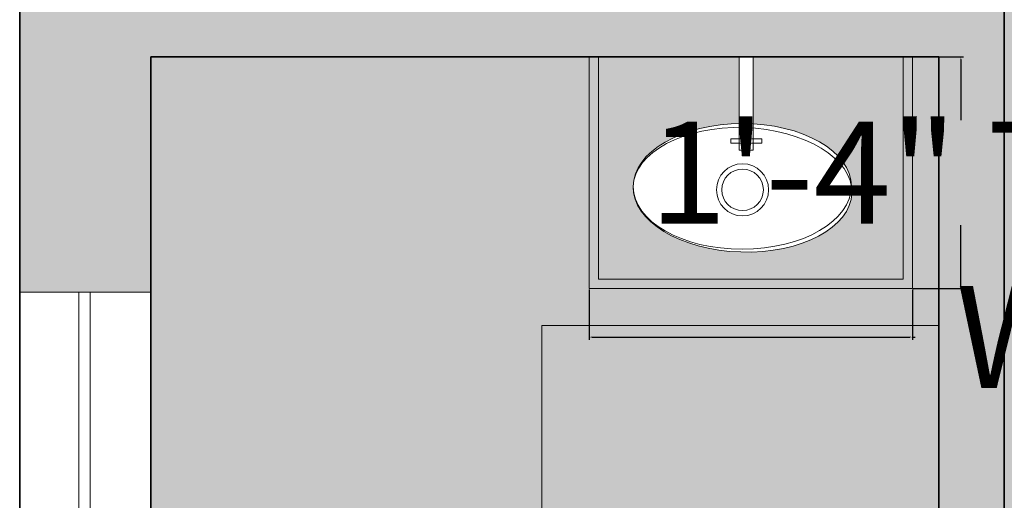
# Model space of a CAD drawing. Units: inches. Extents: x 1316 to 1777, y 813 to 1650.
# Tile 6 of 22: x 1377 to 1445, y 1335 to 1368. Entities that reach past the tile are written whole.
import ezdxf

# ---------------------------------------------------------------- set-up
doc = ezdxf.new("R2010")
doc.units = ezdxf.units.IN
doc.header["$MEASUREMENT"] = 0
for name, color, linetype, lineweight in [('A-ANNO-DIMS', 2, 'Continuous', 18), ('A-FLOR-CASE', 23, 'Continuous', 18), ('A-FLOR-CASE-PATT', 252, 'Continuous', 13), ('A-FLOR-FIXT', 8, 'Continuous', 18), ('A-FLOR-FIXT-PATT', 23, 'Continuous', 13), ('A-WALL-PATT', 250, 'Continuous', 13), ('walls', 250, 'Continuous', 35), ('windows', 141, 'Continuous', 18)]:
    doc.layers.add(name, color=color, linetype=linetype, lineweight=lineweight)
doc.layers.add('A-FLOR-PATT', color=254, linetype='Continuous', lineweight=13, true_color=0xfeeab9)
doc.styles.get("Standard").update_dxf_attribs({"font": 'arial.ttf'})
doc.dimstyles.get("Standard").update_dxf_attribs({"dimtxt": 7, "dimasz": 0.18, "dimexe": 0.18, "dimexo": 0.0625, "dimgap": 0.09, "dimtad": 0, "dimtih": 1, "dimtoh": 1, "dimzin": 0, "dimdsep": 46, "dimlunit": 3, "dimtxsty": 'Standard', "dimcen": 0.09, "dimadec": 0, "dimazin": 0, "dimtfac": 1, "dimtofl": 0, "dimtmove": 0, "dimatfit": 3, "dimfxl": 1, "dimtolj": 1, "dimtzin": 0, "dimarcsym": 0})

# ---------------------------------------------------------------- blocks, each defined once
blk = doc.blocks.new('BASIN-WALL-MOUNT')
for p, q in [((1.14249530725e-05, 15.91430092696169), (1.14249530725e-05, 0.0001979362143629)), ((0.6273383677073526, 15.91430092696169), (0.6273383677073526, 0.658722965959214)), ((10.28959255677932, 9.494232840090262), (10.28959255677932, 15.91430092696191)), ((11.23449039203865, 9.494232840090262), (11.23449039203865, 15.91430092696191)), ((21.53012297768464, 0.658722965959214), (21.53012297768464, 15.91430092696169)), ((22.15516133140068, 0.0001979362143629), (22.15516133140068, 15.91430092696191)), ((9.712388442003657, 10.28665921264746), (11.83648863631629, 10.28665921264746)), ((9.71238844200343, 9.99122808939319), (9.712388442003657, 10.28665921264746)), ((11.83648863631629, 10.28665921264746), (11.83648863631629, 9.99122808939319)), ((11.83648863631629, 9.99122808939319), (9.71238844200343, 9.99122808939319)), ((10.28959255677932, 9.494232840090262), (11.23449039203865, 9.494232840090262)), ((1.14249530725e-05, 0.0001979362143629), (22.15516133140068, 0.0001979362143629)), ((0.6273383677073526, 0.658722965959214), (21.53012297768464, 0.658722965959214))]:
    blk.add_line(p, q)
for radius in [1.786721855987963, 1.786721855987973, 1.426627914243592, 1.426627914243628, 1.42662769250472, 1.426627377330596]:
    blk.add_circle((10.51220414605791, 6.779323088421051), radius)
blk.add_ellipse((10.49584697256341, 7.01803233833516), major_axis=(-7.480193534640648, -0.0164125256646912), ratio=0.5765346257282574)
blk = doc.blocks.new('*D36')
at = {"layer": 'A-ANNO-DIMS', "color": 0, "lineweight": -2, "transparency": 16777216}
for p, q in [((1416.108011424953, 1349.392697936214), (1416.108011424953, 1345.951925450247)), ((1438.2631613314, 1349.392697936214), (1438.2631613314, 1345.951925450247)), ((1416.288011424953, 1346.131925450247), (1438.0831613314, 1346.131925450247)), ((1438.2631613314, 1346.131925450247), (1438.443161331401, 1346.131925450247))]:
    blk.add_line(p, q, dxfattribs=at)
at = {"layer": 'A-ANNO-DIMS', "color": 0, "transparency": 16777216}
for points in [[(1416.288011424953, 1346.161925450247), (1416.288011424953, 1346.101925450247), (1416.108011424953, 1346.131925450247)], [(1438.0831613314, 1346.161925450247), (1438.0831613314, 1346.101925450247), (1438.2631613314, 1346.131925450247)]]:
    blk.add_solid(points, dxfattribs=at)
at = {"layer": 'Defpoints', "color": 0, "transparency": 16777216}
for p in [(1416.108011424953, 1349.455197936214), (1438.2631613314, 1349.455197936214), (1438.2631613314, 1346.131925450247)]:
    blk.add_point(p, dxfattribs=at)
at = {"layer": 'A-ANNO-DIMS', "color": 0, "transparency": 16777216, "insert": (1493.434934864825, 1346.131925450247), "char_height": 7, "attachment_point": 5}
blk.add_mtext('\\A1;WALL BASIN 1\'-10" TYP.', dxfattribs=at)
blk = doc.blocks.new('*D37')
at = {"layer": 'A-ANNO-DIMS', "color": 0, "lineweight": -2, "transparency": 16777216}
for p, q in [((1438.325661331401, 1365.369300926962), (1441.766433817369, 1365.369300926962)), ((1441.586433817368, 1365.189300926962), (1441.586433817368, 1361.018961573471)), ((1441.586433817368, 1349.635197936215), (1441.586433817368, 1353.805537289705)), ((1438.325661331401, 1349.455197936215), (1441.766433817369, 1349.455197936215))]:
    blk.add_line(p, q, dxfattribs=at)
at = {"layer": 'A-ANNO-DIMS', "color": 0, "transparency": 16777216}
for points in [[(1441.556433817369, 1365.189300926962), (1441.616433817368, 1365.189300926962), (1441.586433817368, 1365.369300926962)], [(1441.556433817369, 1349.635197936215), (1441.616433817368, 1349.635197936215), (1441.586433817368, 1349.455197936215)]]:
    blk.add_solid(points, dxfattribs=at)
at = {"layer": 'Defpoints', "color": 0, "transparency": 16777216}
for p in [(1438.263161331401, 1365.369300926962), (1441.586433817368, 1365.369300926962), (1438.263161331401, 1349.455197936215)]:
    blk.add_point(p, dxfattribs=at)
at = {"layer": 'A-ANNO-DIMS', "color": 0, "transparency": 16777216, "insert": (1441.586433817368, 1357.412249431588), "char_height": 7, "attachment_point": 5}
blk.add_mtext('\\A1;1\'-4" TYP.', dxfattribs=at)

msp = doc.modelspace()

# ---------------------------------------------------------------- hatches: boundary and pattern name
at = {"layer": 'A-FLOR-CASE-PATT'}
h = msp.add_hatch(color=256, dxfattribs=at)
h.dxf.hatch_style = 1
h.paths.add_polyline_path([(1412.858226839809, 1346.928610372446), (1440.064450217018, 1346.928610372446), (1440.064450217018, 1365.369300926962), (1438.2631613314, 1365.369300926962), (1438.2631613314, 1349.455197936214), (1416.108011424953, 1349.455197936214), (1416.108011424953, 1365.369300926962), (1386.064450217018, 1365.369300926962), (1386.064450217018, 1245.369300926962), (1412.858226839809, 1245.369300926962)])
h.paths.add_polyline_path([(1409.310422891292, 1332.514765372921, -0.4142135623730951), (1410.210422891292, 1331.614765372921), (1410.210422891292, 1311.814765372921, -0.414213562373094), (1409.310422891292, 1310.914765372921), (1389.51042289129, 1310.914765372921, -0.4142135623730959), (1388.61042289129, 1311.814765372921), (1388.61042289129, 1331.614765372921, -0.4142135623730951), (1389.51042289129, 1332.514765372921)], flags=16)
h.paths.add_polyline_path([(1395.986900854525, 1329.42133126595), (1396.276368249055, 1329.76630507332, -0.0171905986958355), (1396.448908786205, 1329.621893017294), (1396.159470211814, 1329.276953556429, -0.2116405901053515), (1397.086205654243, 1327.18561240685, -0.2564460938474173), (1395.778569555149, 1324.8037474367), (1396.003749512095, 1324.413724310425, -0.0171906504505625), (1395.809203446643, 1324.300687980197), (1395.584072921188, 1324.69062548862, -0.550570801787435), (1391.442799396982, 1327.059740487748), (1390.992413104956, 1327.059740487748, -0.0171907290098312), (1390.991493340996, 1327.284740487748), (1391.441732803486, 1327.284740487748, -0.6105283005508269)], flags=0)
h.paths.add_polyline_path([(1395.838098786515, 1327.18561240685, -1), (1392.688098786514, 1327.18561240685, -1)], flags=0)
h.paths.add_polyline_path([(1394.263098786514, 1328.310612406851, -1), (1394.263098786514, 1326.06061240685, -1)], flags=0)
h.paths.add_polyline_path([(1394.263098786514, 1327.973112406851, -1), (1394.263098786514, 1326.39811240685, -1)], flags=0)
h.paths.add_polyline_path([(1407.468247061996, 1327.18561240685, -0.9779444631718501), (1401.824840804736, 1327.059740487748), (1401.37445451271, 1327.059740487748, -0.0171907290098312), (1401.373534748749, 1327.284740487748), (1401.823774211239, 1327.284740487748, -0.9825922263687022)], flags=0)
h.paths.add_polyline_path([(1406.220140194268, 1327.18561240685, -1), (1403.070140194268, 1327.18561240685, -1)], flags=0)
h.paths.add_polyline_path([(1404.645140194268, 1328.310612406851, -1), (1404.645140194268, 1326.06061240685, -1)], flags=0)
h.paths.add_polyline_path([(1404.645140194268, 1327.973112406851, -1), (1404.645140194268, 1326.39811240685, -1)], flags=0)
h.paths.add_polyline_path([(1400.91382896134, 1321.714765372921, -1), (1397.907016821244, 1321.714765372921, -1)], flags=0)
h.paths.add_polyline_path([(1396.101714535222, 1318.885415367262), (1396.391181929752, 1319.230389174631, -0.0171905986957908), (1396.563722466901, 1319.085977118605), (1396.274283892511, 1318.74103765774, -0.2116405901053402), (1397.201019334939, 1316.649696508162, -0.2564460938474829), (1395.893383235845, 1314.267831538011), (1396.11856319279, 1313.877808411735, -0.0171906504505387), (1395.924017127339, 1313.764772081509), (1395.698886601884, 1314.154709589932, -0.5505708017872751), (1391.557613077679, 1316.523824589059), (1391.107226785653, 1316.523824589059, -0.0171907290098486), (1391.106307021692, 1316.748824589059), (1391.556546484182, 1316.748824589059, -0.6105283005510082)], flags=0)
h.paths.add_polyline_path([(1395.952912467211, 1316.649696508162, -1), (1392.802912467211, 1316.649696508162, -1)], flags=0)
h.paths.add_polyline_path([(1407.468247061996, 1316.611253873528, -0.9779444631716472), (1401.824840804736, 1316.485381954425), (1401.37445451271, 1316.485381954425, -0.0171907290098486), (1401.373534748749, 1316.710381954425), (1401.823774211239, 1316.710381954425, -0.9825922263688615)], flags=0)
h.paths.add_polyline_path([(1394.377912467211, 1317.774696508162, -0.9999999703822144), (1394.377912467211, 1315.524696508162, -0.9999999703822144)], flags=0)
h.paths.add_polyline_path([(1394.377912467211, 1317.437196508162, -1), (1394.377912467211, 1315.862196508162, -1)], flags=0)
h.paths.add_polyline_path([(1406.220140194268, 1316.611253873528, -1), (1403.070140194268, 1316.611253873528, -1)], flags=0)
h.paths.add_polyline_path([(1404.645140194268, 1315.486253873528, -0.9999999703822144), (1404.645140194268, 1317.736253873528, -0.9999999703822144)], flags=0)
h.paths.add_polyline_path([(1404.645140194268, 1317.398753873528, -1), (1404.645140194268, 1315.823753873528, -1)], flags=0)
h.paths.add_polyline_path([(1409.338253781963, 1302.100142632137, -0.4142135623730951), (1410.838253781963, 1300.600142632137), (1410.838253781963, 1270.600142632137, -0.4142135623730951), (1409.338253781963, 1269.100142632137), (1390.338253781963, 1269.100142632137, -0.4142135623730951), (1388.838253781963, 1270.600142632137), (1388.838253781963, 1300.600142632137, -0.4142135623730951), (1390.338253781963, 1302.100142632137)], flags=16)
h.paths.add_polyline_path([(1395.838253781963, 1300.600142632137), (1406.338253781963, 1300.600142632137, -0.4142135623730951), (1409.338253781963, 1297.600142632137), (1409.338253781963, 1289.600142632137, -0.4142135623730951), (1406.338253781963, 1286.600142632137), (1395.838253781963, 1286.600142632137, -0.4142135623730951), (1392.838253781963, 1289.600142632137), (1392.838253781963, 1297.600142632137, -0.4142135623730951)], flags=0)
h.paths.add_polyline_path([(1400.088253781963, 1293.350142632137, -1), (1397.588253781963, 1293.350142632137, -1)], flags=0)
h.paths.add_polyline_path([(1392.338253781963, 1288.600142632137, -1), (1390.338253781963, 1288.600142632137, -1)], flags=0)
h.paths.add_polyline_path([(1393.037126479862, 1286.524525876857), (1399.01645688764, 1282.033156148475), (1398.51645688764, 1281.167130148475), (1391.719002681245, 1284.064804380225, -0.4631994748411593), (1391.203386694108, 1285.500520483254), (1391.606259694108, 1286.198316483253, -0.4369421512224802)], flags=0)
h.paths.add_polyline_path([(1392.338253781963, 1282.600142632137, -1), (1390.338253781963, 1282.600142632137, -1)], flags=0)
h.paths.add_polyline_path([(1400.088253781963, 1277.850142632137, -1), (1397.588253781963, 1277.850142632137, -1)], flags=0)
at = {"layer": 'A-FLOR-FIXT-PATT'}
h = msp.add_hatch(color=256, dxfattribs=at)
h.dxf.hatch_style = 1
h.paths.add_polyline_path([(1438.2631613314, 1365.369300926962), (1437.638122977684, 1365.369300926962), (1437.638122977684, 1350.113722965959), (1416.735338367707, 1350.113722965959), (1416.735338367707, 1365.369300926962), (1416.108011424953, 1365.369300926962), (1416.108011424953, 1349.455197936214), (1438.2631613314, 1349.455197936214)])
h = msp.add_hatch(color=256, dxfattribs=at)
h.dxf.hatch_style = 1
edge = h.paths.add_edge_path()
edge.add_line((1426.397592556779, 1365.369300926962), (1416.735338367707, 1365.369300926962))
edge.add_line((1416.735338367707, 1365.369300926962), (1416.735338367707, 1350.113722965959))
edge.add_line((1416.735338367707, 1350.113722965959), (1437.638122977684, 1350.113722965959))
edge.add_line((1437.638122977684, 1350.113722965959), (1437.638122977684, 1365.369300926962))
edge.add_line((1437.638122977684, 1365.369300926962), (1427.342490392038, 1365.369300926962))
edge.add_line((1427.342490392038, 1365.369300926962), (1427.342490392038, 1360.765644863863))
edge.add_ellipse((1426.603846972563, 1356.473032338335), major_axis=(-7.480193534640648, -0.0164125256646912), ratio=0.5765346257282575, start_angle=180, end_angle=260.11083298804067, ccw=False)
edge.add_ellipse((1426.620204146058, 1356.234323088421), major_axis=(7.496550708135166, -0.2222967242493548), ratio=0.5689904069289865, start_angle=-180, end_angle=3.6561733604243045, ccw=False)
edge.add_ellipse((1426.603846972563, 1356.473032338335), major_axis=(-7.480193534640648, -0.0164125256646912), ratio=0.5765346257282575, start_angle=272.6136539907866, end_angle=360, ccw=False)
edge.add_line((1426.397592556779, 1360.783698373135), (1426.397592556779, 1365.369300926962))
at = {"layer": 'A-FLOR-PATT'}
h = msp.add_hatch(color=256, dxfattribs=at)
h.dxf.hatch_style = 1
h.paths.add_polyline_path([(1567.673142217696, 1281.369300926962), (1651.673142217696, 1281.369300926962), (1651.673142217696, 1365.369300926962), (1597.673142217696, 1365.369300926962), (1597.673142217696, 1429.869300926962), (1570.345136951899, 1429.869300926962), (1570.345136951899, 1471.869300926962), (1510.345136951899, 1471.869300926962), (1510.345136951899, 1429.869300926962), (1444.564450217018, 1429.869300926962), (1444.564450217018, 1322.882360660317), (1444.564450217018, 1300.087519887597), (1510.564450217018, 1300.087519887597), (1510.564450217018, 1295.093869264817), (1510.564450217018, 1240.869300926962), (1386.064450217018, 1240.869300926962), (1386.064450217018, 1171.184826128129), (1400.961298831769, 1171.184826128129), (1400.961298831769, 1106.74181853581), (1386.064450217018, 1106.74181853581), (1386.064450217018, 1072.869300926962), (1510.564450217018, 1072.869300926962), (1510.564450217018, 1040.172951843256), (1541.068383692007, 1040.172951843256, -0.367085007058701), (1572.764174999282, 1069.546549507821), (1572.764174999282, 1069.578525976929), (1574.225256623933, 1069.578525976929), (1574.225256623933, 1040.172951843256), (1616.037285953149, 1040.172951843256), (1616.037285953149, 1086.627161740109), (1616.037285953149, 1103.704513499145), (1613.066060418845, 1105.234780569291), (1616.037285953149, 1106.685539866415), (1616.037285953149, 1123.869300926962), (1567.673142217696, 1123.869300926962)])
h.paths.add_polyline_path([(1508.987494855724, 1198.018101264616), (1511.117481528599, 1198.018101264616), (1511.117481528599, 1200.148087937491), (1532.594847146751, 1200.148087937491), (1532.594847146751, 1198.018101264616), (1534.724833819626, 1198.018101264616), (1534.724833819626, 1176.008238978245), (1530.464860473877, 1176.008238978245), (1530.464860473877, 1176.71823453587), (1513.247468201473, 1176.71823453587), (1513.247468201473, 1176.008238978245), (1508.987494855724, 1176.008238978245)], flags=16)
h.paths.add_polyline_path([(1505.978911344017, 1151.314990471522), (1521.503967005494, 1151.314990471522), (1521.503967005494, 1123.622553675171), (1505.978911344017, 1123.622553675171)], flags=16)
h.paths.add_polyline_path([(1507.734238645614, 1150.100746953806, -1), (1506.932299902515, 1150.100746953806, -1)], flags=0)
h.paths.add_polyline_path([(1512.288074001727, 1138.353334368216), (1512.279600715468, 1138.392440283947), (1512.219350358134, 1138.376242249414)], flags=0)
h.paths.add_polyline_path([(1511.538708600003, 1138.926307509397), (1511.801586230713, 1138.967144364025), (1511.816822451641, 1139.269704188439), (1511.606794574277, 1139.246286533845)], flags=0)
h.paths.add_polyline_path([(1513.744555260512, 1140.234298321423), (1513.680232363733, 1139.885116881769), (1514.013725426534, 1140.045442118172), (1513.85452204526, 1140.307851476896)], flags=0)
h.paths.add_polyline_path([(1513.759454991183, 1139.088508933479), (1514.004707571892, 1139.255238426424), (1513.806733823314, 1139.482778214552), (1513.564128907831, 1139.327271464974)], flags=0)
h.paths.add_polyline_path([(1514.219475210051, 1138.385213274156), (1514.335730050378, 1138.330012877603), (1514.544443105969, 1138.319719602207), (1514.802071501717, 1138.873746829037), (1514.451386945615, 1138.715560522777)], flags=0)
h.paths.add_polyline_path([(1514.576784523415, 1137.439218133731), (1514.572807725035, 1137.400121795131), (1514.699202201671, 1137.400121795131), (1514.696265725507, 1137.401958254237)], flags=0)
h.paths.add_polyline_path([(1512.259630054145, 1136.199252443718), (1512.198645006043, 1136.399020086717), (1512.031969302785, 1136.324884611944), (1512.095408670439, 1136.101205019573), (1512.257489338984, 1136.192116726515)], flags=0)
h.paths.add_polyline_path([(1512.643663084783, 1137.273739653883), (1512.355504649132, 1137.230281342332), (1512.431954114942, 1137.048783229095), (1512.702875297586, 1137.092989450977)], flags=0)
h.paths.add_polyline_path([(1513.048588650928, 1137.592520798729), (1512.979298324136, 1137.799799709794), (1512.842806872769, 1137.757466697763), (1512.887278702865, 1137.556025839099)], flags=0)
h.paths.add_polyline_path([(1513.269281623239, 1138.555876366321), (1513.570749546786, 1137.962332598873), (1513.458764523686, 1136.814048268166), (1513.212081965274, 1137.877990637943), (1513.032322366809, 1138.442602014432)], flags=0)
h.paths.add_polyline_path([(1514.891020715756, 1136.377090047208), (1514.695899864911, 1136.400535518201), (1514.682939550409, 1136.245500587688), (1514.870369662043, 1136.165423867704)], flags=0)
h.paths.add_polyline_path([(1514.142311807212, 1137.292647657223), (1514.047049214511, 1136.74320071616), (1514.270411313405, 1136.750949401328), (1514.327746372416, 1137.265481105849)], flags=0)
h.paths.add_polyline_path([(1515.361925908058, 1138.975942407129), (1515.333738674027, 1138.638448296537), (1515.595602136156, 1138.588081597507), (1515.627104749056, 1138.931608018565)], flags=0)
h.paths.add_polyline_path([(1537.284795120854, 1177.912388692567), (1537.994790678479, 1177.912388692567), (1537.994790678479, 1195.129780964971), (1537.284795120854, 1195.129780964971), (1537.284795120854, 1199.38975431072), (1559.294657407225, 1199.38975431072), (1559.294657407225, 1197.259767637845), (1561.4246440801, 1197.259767637845), (1561.4246440801, 1175.782402019693), (1559.294657407225, 1175.782402019693), (1559.294657407225, 1173.652415346818), (1559.378615070445, 1173.652415346818), (1559.378615070445, 1171.514303738793), (1561.51672667847, 1171.514303738793), (1561.51672667847, 1098.818509065945), (1559.378615070445, 1098.818509065945), (1559.378615070445, 1096.68039745792), (1537.284795120854, 1096.68039745792), (1537.284795120854, 1100.95662067397), (1537.997498990196, 1100.95662067397), (1537.997498990196, 1169.376192130768), (1537.284795120854, 1169.376192130768), (1537.284795120854, 1173.652415346818)], flags=16)
h.paths.add_polyline_path([(1518.623279367581, 1345.565265318288), (1519.133216999197, 1345.479657117201), (1519.133247129367, 1345.484585273925), (1518.623292796693, 1345.567461813277)], flags=16)
h.paths.add_polyline_path([(1518.798043157878, 1374.150014517315), (1519.307980789494, 1374.064406316228), (1519.308010919664, 1374.069334472953), (1518.79805658699, 1374.152211012305)], flags=16)
h.paths.add_polyline_path([(1537.763945546351, 1413.501272593833), (1537.678419015976, 1412.991334462891), (1537.683273643974, 1412.991304782267), (1537.76615767817, 1413.501259069119)], flags=16)
h.paths.add_polyline_path([(1572.904903294898, 1373.821409718101), (1573.926762419731, 1373.974678074354), (1574.026627442758, 1390.308820473798), (1573.007147246318, 1390.474521481455), (1573.006718884663, 1390.474591095266)], flags=16)
h.paths.add_polyline_path([(1572.730139504601, 1345.236660519073), (1573.751998629434, 1345.389928875326), (1573.851863652461, 1361.72407127477), (1572.832383456021, 1361.889772282427), (1572.831955094366, 1361.889841896238)], flags=16)
h.paths.add_polyline_path([(1537.210658487583, 1322.64259197221), (1537.363943428096, 1321.620732745983), (1553.69808582754, 1321.520867722956), (1553.863838585734, 1322.540776390265)], flags=16)
h.paths.add_polyline_path([(1535.907853535946, 1331.328394679552), (1527.214399285865, 1331.381545435045), (1527.663791889487, 1404.885186232545), (1564.415612288236, 1404.660489930734), (1563.966219684615, 1331.156849133235), (1555.272745017813, 1331.210000013553), (1553.946716560728, 1323.050730714162), (1537.134020158137, 1323.153521560007)], flags=16)
h.paths.add_polyline_path([(1536.149948378398, 1336.502989385165), (1536.235164066325, 1337.571577967879), (1536.323287084786, 1338.628101895201), (1536.410786509507, 1339.662781903015), (1536.494625364907, 1340.6698173033), (1536.573878305868, 1341.65983134291), (1536.648126641431, 1342.647834135966), (1536.716972722469, 1343.648937760143), (1536.780017027388, 1344.677948027938), (1536.836830656389, 1345.749875115879), (1536.91349345135, 1347.47536960008), (1536.930181129876, 1348.082213381731), (1536.86671979596, 1346.313806322279), (1536.754065794645, 1344.188314997416), (1536.618602559507, 1342.21851898877), (1536.494625364906, 1340.669817303289), (1536.410786509508, 1339.662781903024), (1536.323287084785, 1338.628101895196), (1536.235164066325, 1337.571577967878), (1536.149948378398, 1336.502989385167), (1536.071202820108, 1335.432319400725), (1536.002480605875, 1334.369653419014), (1535.917201218224, 1332.754159960459), (1535.909282823342, 1332.307756473361), (1535.96435308899, 1333.780079645636), (1536.071202820108, 1335.432319400726)], flags=0)
h.paths.add_polyline_path([(1540.411728678358, 1338.345220732376), (1540.538507986221, 1339.036732867615), (1540.667450686668, 1339.758144792479), (1540.798139602249, 1340.51803480286), (1540.930104638842, 1341.324675241543), (1541.06290820131, 1342.186644529235), (1541.195663950278, 1343.109256879628), (1541.325751198274, 1344.084667215432), (1541.450112594895, 1345.102072455087), (1541.565699126105, 1346.150363189455), (1541.669432399664, 1347.218634373414), (1541.758274858692, 1348.295980712192), (1541.829158319786, 1349.371497098253), (1541.87902418423, 1350.434176273261), (1541.905658245644, 1351.475864398132), (1541.910264078201, 1352.499718972741), (1541.894848813054, 1353.511751165878), (1541.861450207875, 1354.517971959091), (1541.812104772023, 1355.524188157142), (1541.748831093802, 1356.536615043187), (1541.673675267255, 1357.560957271187), (1541.551221046702, 1359.062282646612), (1541.495486505545, 1359.670454934914), (1541.588655256529, 1358.603328035907), (1541.721318618915, 1356.976835527602), (1541.846114060333, 1354.980013725856), (1541.912433480836, 1352.981966815021), (1541.903299375855, 1350.951498912638), (1541.805645357175, 1348.870418133965), (1541.627733180341, 1346.712969607265), (1541.39605931794, 1344.611846225434), (1541.135168242209, 1342.655652549989), (1540.871929016276, 1340.947082961546), (1540.617179283622, 1339.465841984599), (1540.411728678363, 1338.345220732389), (1540.287580984743, 1337.67502977883), (1540.166494164132, 1337.01788791383), (1540.048925605183, 1336.365114503449), (1539.936674201221, 1335.710368832696), (1539.836864251217, 1335.055036635329), (1539.758020939376, 1334.402536924379), (1539.708629238703, 1333.756391050932), (1539.697173498044, 1333.120018277682), (1539.75093556766, 1332.162191347439), (1539.822087714565, 1331.89006440645), (1539.690956844971, 1332.774679737417), (1539.713650637448, 1334.035332547662), (1539.86680860596, 1335.30285325234), (1540.085210789094, 1336.576760560778), (1540.287580984743, 1337.67502977883)], flags=0)
h.paths.add_polyline_path([(1545.598581542273, 1331.583674047033), (1545.601408931398, 1331.616855477121), (1545.614142276281, 1331.689058908809), (1545.736718477884, 1332.197227143153), (1545.766951209007, 1332.331509735297), (1545.840044120643, 1332.681341212682), (1545.924609388668, 1333.114205605127), (1546.015565858785, 1333.613901317454), (1546.107830504227, 1334.163920489319), (1546.196310713542, 1334.747857411176), (1546.27592408412, 1335.349306311069), (1546.341588213349, 1335.951861417042), (1546.388220074462, 1336.539014868746), (1546.411904372759, 1337.098233262493), (1546.413511757999, 1337.631655211558), (1546.395048737181, 1338.145189796344), (1546.358553067975, 1338.644847998394), (1546.30606313221, 1339.136742887642), (1546.239595021565, 1339.626681393686), (1546.161196702551, 1340.120674435653), (1546.072884891005, 1340.624631031533), (1545.887738197254, 1341.63015699768), (1545.717659533451, 1342.62070013092), (1545.546853733249, 1343.94500888803), (1545.431881256549, 1345.533720124316), (1545.403899849759, 1347.401905451854), (1545.417510423816, 1348.013069267128), (1545.410556413592, 1346.957478372932), (1545.425070640934, 1345.988432507364), (1545.462877367243, 1345.105410056077), (1545.521092971858, 1344.300975918152), (1545.595702123642, 1343.566272620922), (1545.68263719895, 1342.892238827028), (1545.777872657803, 1342.270017126221), (1545.877351709551, 1341.690648207114), (1545.977037981224, 1341.145172633476), (1546.133225269608, 1340.296924301995), (1546.32712189736, 1339.07516870602), (1546.43378476773, 1337.614859053002), (1546.377188266119, 1336.278538916938), (1546.246417261819, 1335.078542247844), (1546.032296532176, 1333.665423983985), (1545.840044120643, 1332.681341212682), (1545.766951209007, 1332.331509735297)], flags=0)
h.paths.add_polyline_path([(1551.802739251137, 1337.655775652498), (1551.96257269545, 1338.249893918501), (1552.102195298518, 1338.801154932478), (1552.224958021371, 1339.338328209144), (1552.330696453755, 1339.864579612065), (1552.418402861907, 1340.377056720641), (1552.487067639598, 1340.872600849098), (1552.535672844225, 1341.34835963925), (1552.563199284875, 1341.801276556129), (1552.568639227787, 1342.228499179132), (1552.550972857889, 1342.626868884903), (1552.509678498417, 1342.994551203202), (1552.446288501197, 1343.33337442512), (1552.362792521005, 1343.646491244529), (1552.261208966661, 1343.936747902882), (1552.143557495304, 1344.207194818415), (1552.011836098078, 1344.460678357413), (1551.868075265113, 1344.700350964085), (1551.746105860759, 1344.881722683215), (1550.887297650741, 1346.05192221882), (1550.42788872704, 1347.125680184261), (1550.183287427721, 1348.353333686171), (1550.047936052465, 1349.632359022536), (1549.978096005541, 1351.223542107026), (1549.974102148838, 1353.140827975589), (1549.989226669163, 1353.748427546368), (1549.975058438592, 1352.681752708607), (1549.977087298692, 1351.70778065901), (1549.995607655661, 1350.824569845699), (1550.030618304039, 1350.026913573531), (1550.082058657804, 1349.309911787039), (1550.149928759809, 1348.668561967865), (1550.234168024029, 1348.097964060535), (1550.334775869163, 1347.593013458303), (1550.451691709185, 1347.148810105696), (1550.584412233058, 1346.759844100773), (1550.73038050297, 1346.418678345312), (1550.88655602074, 1346.117266144286), (1551.049909745336, 1345.847764917032), (1551.217401178577, 1345.602127968521), (1551.385990446439, 1345.372410692116), (1551.55262809021, 1345.150770631988), (1552.000038284146, 1344.537104232464), (1552.453505275841, 1343.494713960715), (1552.591463897673, 1342.266339273388), (1552.508711326437, 1340.904737898757), (1552.245597777252, 1339.367339734202), (1551.924893638995, 1338.101128644033), (1551.618511514029, 1336.984114361546), (1551.405674157756, 1336.200020283199), (1551.009764092749, 1334.698598399404), (1550.877399289293, 1334.154667887629), (1551.263664389663, 1335.676855458292), (1551.618511514027, 1336.984114361536)], flags=0)
h.paths.add_polyline_path([(1558.642358998526, 1348.348341932098), (1558.795153425402, 1348.811416841303), (1558.918173552255, 1349.215358215379), (1559.008026171039, 1349.574581801048), (1559.061298904339, 1349.903707646641), (1559.075825921932, 1350.214183320864), (1559.054343192669, 1350.505992096326), (1559.00083323259, 1350.775944766007), (1558.919250427844, 1351.021260663692), (1558.81356708563, 1351.238750644777), (1558.687756761463, 1351.425429741436), (1558.545793010855, 1351.578312985846), (1558.391628971643, 1351.694415535011), (1558.228764001313, 1351.771674150153), (1558.05869086465, 1351.812121548804), (1557.882428128411, 1351.81871217754), (1557.700994359352, 1351.79440048294), (1557.515397915392, 1351.742140973996), (1557.326668820441, 1351.665092211649), (1557.135793766425, 1351.566004652943), (1556.943823194933, 1351.44803673399), (1556.751584825563, 1351.314654529213), (1556.741969848742, 1351.307485185875), (1556.174649390243, 1350.878470713214), (1555.982386678774, 1350.741107061228), (1555.790208852573, 1350.61762743028), (1555.103431920574, 1350.247624890473), (1554.019478994433, 1350.696346369238), (1553.658410413117, 1351.73359972735), (1553.592207666961, 1352.861368347784), (1553.704659497418, 1354.248209262139), (1553.753119918252, 1354.656598557367), (1553.684819216316, 1354.00352392911), (1553.637913725648, 1353.425049987856), (1553.614699631385, 1352.917691559993), (1553.614827379228, 1352.476039895736), (1553.637249468889, 1352.094077959223), (1553.680938817757, 1351.765788589762), (1553.744858758541, 1351.485256777466), (1553.82798220863, 1351.246465361642), (1553.929261667735, 1351.043397306428), (1554.04767130156, 1350.870239627912), (1554.182026927633, 1350.721997047951), (1554.330490954936, 1350.598680801359), (1554.491077653114, 1350.501119766308), (1554.661792955443, 1350.430449148551), (1554.840661964566, 1350.387599852234), (1555.02568040492, 1350.373707145527), (1555.214873379145, 1350.389701932573), (1555.406255781046, 1350.436515179933), (1555.598153361026, 1350.514157123772), (1555.790208852573, 1350.61762743028), (1555.982386678773, 1350.741107061227), (1556.174649390244, 1350.878470713214), (1556.366961410069, 1351.02389934801), (1556.559285288865, 1351.171267662216), (1556.751584825563, 1351.314654529213), (1556.943823194933, 1351.44803673399), (1557.135793766425, 1351.566004652943), (1557.326668820441, 1351.665092211648), (1558.042515074605, 1351.95733685961), (1558.893728230531, 1351.316279335487), (1559.136865914879, 1350.089672795452), (1558.886015641058, 1349.086793457618), (1558.642358998525, 1348.348341932093), (1558.463193064356, 1347.811615590227), (1558.261048830942, 1347.186822068983), (1558.03933929985, 1346.459443408408), (1557.677450203418, 1345.174834336041), (1557.548968991007, 1344.635807724703), (1557.908545731516, 1346.030339390738), (1558.328508124364, 1347.408140702653)], flags=0)
h.paths.add_polyline_path([(1562.145123345359, 1353.919129120074), (1562.250304117219, 1354.679787637482), (1562.34093833006, 1355.343853771733), (1562.416101040585, 1355.923686334763), (1562.475035862508, 1356.430826370303), (1562.517611688201, 1356.872216949942), (1562.54387555173, 1357.25388122627), (1562.553854069482, 1357.581842476714), (1562.547593651368, 1357.862021765479), (1562.525120913776, 1358.10044236999), (1562.486482890773, 1358.30312744284), (1562.431704950433, 1358.475896084676), (1562.361155192264, 1358.623850655281), (1562.276503898586, 1358.748001864806), (1562.179752001843, 1358.848337479786), (1562.072869183806, 1358.924743365611), (1561.957877418753, 1358.977309252376), (1561.836746388454, 1359.005921005473), (1561.71148785835, 1359.010668417409), (1561.584092552045, 1358.991539317136), (1561.456045120288, 1358.949239273116), (1561.341584300566, 1358.895014406292), (1560.779829007024, 1358.553784684453), (1560.630616275888, 1358.472819004295), (1560.474487483611, 1358.402819474164), (1560.311154867376, 1358.348484094885), (1559.637466910391, 1358.206630908504), (1558.973121038646, 1358.903907683205), (1558.815552073528, 1360.002456271339), (1558.803942930122, 1361.236291863163), (1558.829841213422, 1361.673699707903), (1558.80694301689, 1360.917438550413), (1558.812784665874, 1360.296580130481), (1558.845278068372, 1359.795210830316), (1558.902335132382, 1359.397417032129), (1558.981856932905, 1359.087183092155), (1559.081756002095, 1358.848697480995), (1559.199942999639, 1358.66584240408), (1559.334180223548, 1358.524951186848), (1559.481597784608, 1358.420834672959), (1559.639186392453, 1358.350550586885), (1559.803946965561, 1358.311156590683), (1559.97287021357, 1358.299710408824), (1560.142945597805, 1358.313065589002), (1560.311154867377, 1358.348484094885), (1560.474487483611, 1358.402819474164), (1560.630616275888, 1358.472819004295), (1560.779829007024, 1358.553784684454), (1560.923096183733, 1358.640810155187), (1561.061387688574, 1358.728886968651), (1561.195663195268, 1358.813006739421), (1561.382100208996, 1358.919625179564), (1561.341584300566, 1358.895014406292), (1561.972476451099, 1359.193894345525), (1562.53631106285, 1358.366963698877), (1562.559911530188, 1357.31074636116), (1562.455247211757, 1356.225674176933), (1562.323097858171, 1355.206225864646), (1562.145123345359, 1353.91912912008), (1562.026320333625, 1353.049417319218), (1561.815039989057, 1351.456922136686), (1561.751502783429, 1350.932786338753), (1561.948339842468, 1352.478551712307)], flags=0)
h.paths.add_polyline_path([(1572.764174999282, 1069.546549507821, 0.3670850070587006), (1541.068383692007, 1040.172951843256), (1572.764174999282, 1040.172951843256)], flags=17)
h.paths.add_polyline_path([(1572.764174999282, 1040.172951843256), (1541.068383692007, 1040.172951843256, 0.0299535364659094), (1540.829105203347, 1036.182374556343), (1540.829105203347, 1031.172951843255), (1574.225256623933, 1031.172951843255), (1574.225256623933, 1036.182374556343), (1572.764174999282, 1036.182374556343)])
h = msp.add_hatch(color=256, dxfattribs=at)
h.dxf.hatch_style = 1
h.paths.add_polyline_path([(1506.064450217018, 1295.093869264817), (1444.564450217018, 1295.093869264817), (1444.564450217018, 1322.882360660317), (1440.064450217018, 1322.882360660317), (1440.064450217018, 1346.928610372446), (1412.858226839809, 1346.928610372446), (1412.858226839809, 1245.369300926962), (1506.064450217018, 1245.369300926962)])
h.paths.add_polyline_path([(1484.664907055627, 1269.305233675322), (1504.590417462121, 1269.305233675322), (1504.590417462121, 1245.841035562835), (1484.664907055627, 1245.841035562835)], flags=16)
h.paths.add_polyline_path([(1510.564450217018, 1300.087519887597), (1444.564450217018, 1300.087519887597), (1444.564450217018, 1295.093869264817), (1506.064450217018, 1295.093869264817), (1510.564450217018, 1295.093869264817)])
at = {"layer": 'A-WALL-PATT'}
h = msp.add_hatch(color=256, dxfattribs=at)
h.dxf.hatch_style = 1
h.paths.add_polyline_path([(1713.173142217696, 1281.369300926962), (1656.173142217696, 1281.369300926962), (1656.173142217696, 1298.257717658217), (1651.673142217696, 1298.257717658217), (1651.673142217696, 1281.369300926962), (1567.673142217696, 1281.369300926962), (1567.673142217696, 1266.995117174766), (1572.173142217695, 1266.995117174766), (1572.173142217695, 1276.869300926963), (1704.173142217696, 1276.869300926962), (1704.173142217696, 1132.869300926962), (1608.640148269009, 1132.869300926962), (1608.640148269009, 1123.869300926962), (1704.173142217696, 1123.869300926962), (1704.173142217696, 1040.172951843256), (1652.868762127258, 1040.172951843256), (1652.868762127258, 1031.172951843254), (1713.173142217696, 1031.172951843253), (1713.173142217696, 1040.172951843256)])
h.paths.add_polyline_path([(1572.173142217696, 1237.954794134253), (1567.673142217696, 1237.954794134253), (1567.673142217696, 1123.869300926962), (1583.145592691861, 1123.869300926962), (1583.145592691861, 1132.869300926963), (1572.173142217696, 1132.869300926963)], flags=17)
h.paths.add_polyline_path([(1510.345136951899, 1566.369300926962), (1524.170902149835, 1566.369300926962), (1524.170902149835, 1571.984613741441), (1524.170902149835, 1575.369300926961), (1445.954793584458, 1575.369300926961), (1445.954793584458, 1566.369300926962), (1505.845136951899, 1566.369300926962), (1505.845136951899, 1469.591483064839), (1510.345136951899, 1469.591483064839), (1510.345136951899, 1471.869300926962), (1529.081211183796, 1471.869300926962), (1529.081211183796, 1476.369300926962), (1510.345136951899, 1476.369300926962)])
h.paths.add_polyline_path([(1609.722471703215, 1575.369300926961), (1545.118796217357, 1575.369300926961), (1545.118796217357, 1566.369300926962), (1570.345136951899, 1566.369300926962), (1570.345136951899, 1476.369300926962), (1562.477362604382, 1476.369300926962), (1562.477362604382, 1471.869300926962), (1570.345136951899, 1471.869300926962), (1570.345136951899, 1469.591483064839), (1574.845136951899, 1469.591483064839), (1574.845136951899, 1566.369300926962), (1609.722471703215, 1566.369300926962)])
h.paths.add_polyline_path([(1713.173142217696, 1575.369300926961), (1655.232651300773, 1575.369300926961), (1655.232651300773, 1566.369300926962), (1704.173142217696, 1566.369300926962), (1704.173142217696, 1434.369300926962), (1574.845136951899, 1434.369300926962), (1574.845136951899, 1440.551160024325), (1574.701185407976, 1440.551160024325), (1570.345136951899, 1440.551160024325), (1570.345136951899, 1429.869300926962), (1597.673142217696, 1429.869300926962), (1597.673142217696, 1408.281186528541), (1602.173142217695, 1408.281186528541), (1602.173142217695, 1429.869300926962), (1704.173142217696, 1429.869300926962), (1704.173142217696, 1410.703982852585), (1707.374745037781, 1410.703982852585), (1713.173142217696, 1410.703982852585)])
h.paths.add_polyline_path([(1713.173142217696, 1383.675544097327), (1704.173142217696, 1383.675544097327), (1704.173142217696, 1369.869300926962), (1602.173142217696, 1369.869300926962), (1602.173142217695, 1379.240863488028), (1597.673142217696, 1379.240863488028), (1597.673142217696, 1365.369300926962), (1713.173142217696, 1365.369300926962)])
h.paths.add_polyline_path([(1444.564450217018, 1429.869300926962), (1510.345136951899, 1429.869300926962), (1510.345136951899, 1440.551160024325), (1505.845136951899, 1440.551160024325), (1505.845136951899, 1434.369300926962), (1386.064450217018, 1434.369300926961), (1386.064450217018, 1566.369300926962), (1400.4446139869, 1566.369300926962), (1400.4446139869, 1575.369300926961), (1377.064450217018, 1575.369300926961), (1377.064450217018, 1412.813262305812), (1380.508552477466, 1412.813262305812), (1386.064450217018, 1412.813262305812), (1386.064450217018, 1429.869300926962), (1440.064450217018, 1429.869300926962), (1440.064450217018, 1401.229090636953), (1444.564450217018, 1401.229090636953)])
h.paths.add_polyline_path([(1444.564450217018, 1372.18876759644), (1440.064450217018, 1372.18876759644), (1440.064450217018, 1369.869300926962), (1386.064450217018, 1369.869300926962), (1386.064450217018, 1378.757622609401), (1377.064450217018, 1378.757622609401), (1377.064450217018, 1349.201183977028), (1381.117947355797, 1349.201183977028), (1386.064450217018, 1349.201183977028), (1386.064450217018, 1365.369300926962), (1440.064450217018, 1365.369300926962), (1440.064450217018, 1322.882360660317), (1444.564450217018, 1322.882360660317)])
h.paths.add_polyline_path([(1510.564450217018, 1295.093869264817), (1506.064450217018, 1295.093869264817), (1506.064450217018, 1245.369300926962), (1386.064450217018, 1245.369300926962), (1386.064450217018, 1272.58216425724), (1377.064450217018, 1272.58216425724), (1377.064450217018, 1212.904590025772), (1380.100240558029, 1212.904590025772), (1386.064450217018, 1212.904590025772), (1386.064450217018, 1240.869300926962), (1510.564450217018, 1240.869300926962)])
h.paths.add_polyline_path([(1386.064450217018, 1163.761289951094), (1377.064450217018, 1163.761289951094), (1377.064450217018, 1063.869300926961), (1419.36334498438, 1063.869300926961), (1419.36334498438, 1072.869300926962), (1386.064450217018, 1072.869300926962)])
h.paths.add_polyline_path([(1510.564450217018, 1072.869300926962), (1469.381492401113, 1072.869300926962), (1469.381492401113, 1063.869300926961), (1501.564450217018, 1063.869300926962), (1501.564450217018, 1033.022564166395), (1501.564450217018, 1031.172951843256), (1540.829105203347, 1031.172951843255), (1540.829105203347, 1036.182374556343, -0.0299535364659092), (1541.068383692007, 1040.172951843256), (1510.564450217018, 1040.172951843256)])
h.paths.add_polyline_path([(1607.368796217357, 1040.172951843256), (1574.225256623933, 1040.172951843256), (1574.225256623933, 1036.182374556343), (1574.225256623933, 1031.172951843255), (1607.368796217357, 1031.172951843254)], flags=17)
h.paths.add_polyline_path([(1637.054389108292, 1040.172951843256), (1624.70577568894, 1040.172951843256), (1624.70577568894, 1031.172951843254), (1637.054389108293, 1031.172951843254)], flags=17)

# ---------------------------------------------------------------- linework, layer by layer
at = {"layer": 'A-FLOR-CASE'}
for p, q in [((1440.064450217018, 1346.928610372446), (1412.858226839809, 1346.928610372446)), ((1412.858226839809, 1346.928610372446), (1412.858226839809, 1245.369300926962))]:
    msp.add_line(p, q, dxfattribs=at)
at = {"layer": 'A-FLOR-FIXT', "extrusion": (0, 0, -0.9999999999999998)}
msp.add_ellipse((1426.620204146058, 1356.234323088421), major_axis=(7.496550708135166, -0.2222967242493548), ratio=0.5689904069289865, dxfattribs=at)
at = {"layer": 'walls'}
for p, q in [((1377.064450217018, 1575.369300926961), (1377.064450217018, 953.6889813170072)), ((1444.564450217018, 1429.869300926962), (1444.564450217018, 1322.882360660317)), ((1386.064450217018, 1365.369300926962), (1440.064450217018, 1365.369300926962)), ((1386.064450217018, 1365.369300926962), (1386.064450217018, 1245.369300926962)), ((1440.064450217018, 1365.369300926962), (1440.064450217018, 1322.882360660317))]:
    msp.add_line(p, q, dxfattribs=at)
at = {"layer": 'windows'}
for p, q in [((1377.064450217018, 1349.201183977028), (1386.064450217018, 1349.201183977028)), ((1377.064450217018, 1344.130177497399), (1377.064450217018, 1349.201183977028)), ((1377.064450217018, 1349.201183977028), (1381.117947355797, 1349.201183977028)), ((1381.117947355797, 1349.201183977028), (1381.117947355797, 1272.58216425724)), ((1381.904112948374, 1272.58216425724), (1381.904112948374, 1349.201183977028)), ((1386.064450217018, 1349.201183977028), (1386.064450217018, 1272.58216425724)), ((1377.064450217018, 1272.58216425724), (1377.064450217018, 1344.130177497399))]:
    msp.add_line(p, q, dxfattribs=at)

# ---------------------------------------------------------------- block references
at = {"layer": 'A-FLOR-FIXT'}
msp.add_blockref('BASIN-WALL-MOUNT', (1416.108, 1349.455), dxfattribs=at)

# ---------------------------------------------------------------- dimensions: what is measured, and where the dimension line sits
at = {"layer": 'A-ANNO-DIMS'}
dim = msp.add_linear_dim(base=(1438.2631613314, 1346.131925450247), p1=(1416.108011424953, 1349.455197936214), p2=(1438.2631613314, 1349.455197936214), text='WALL BASIN <> TYP.', dimstyle='Standard', override={"dimdec": 1, "dimlfac": 1, "dimrnd": 0, "dimzin": 1, "dimdsep": 46, "dimlunit": 4, "dimfrac": 2}, dxfattribs=at)
dim.commit()
dim.dimension.update_dxf_attribs({"geometry": '*D36', "text_midpoint": (1493.434934864825, 1346.131925450247)})
dim = msp.add_linear_dim(base=(1441.586433817368, 1365.369300926962), p1=(1438.2631613314, 1349.455197936214), p2=(1438.2631613314, 1365.369300926962), angle=90, text='<> TYP.', dimstyle='Standard', override={"dimdec": 1, "dimlfac": 1, "dimrnd": 0, "dimzin": 1, "dimdsep": 46, "dimlunit": 4, "dimfrac": 2}, dxfattribs=at)
dim.commit()
dim.dimension.update_dxf_attribs({"geometry": '*D37', "text_midpoint": (1441.586433817368, 1357.412249431588)})

doc.saveas('drawing.dxf')
